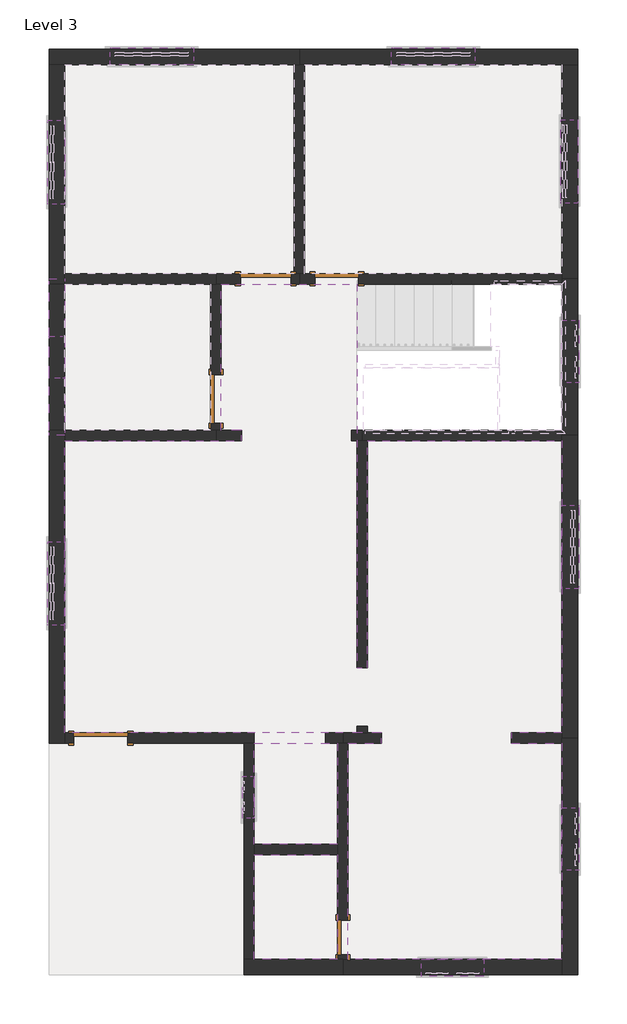
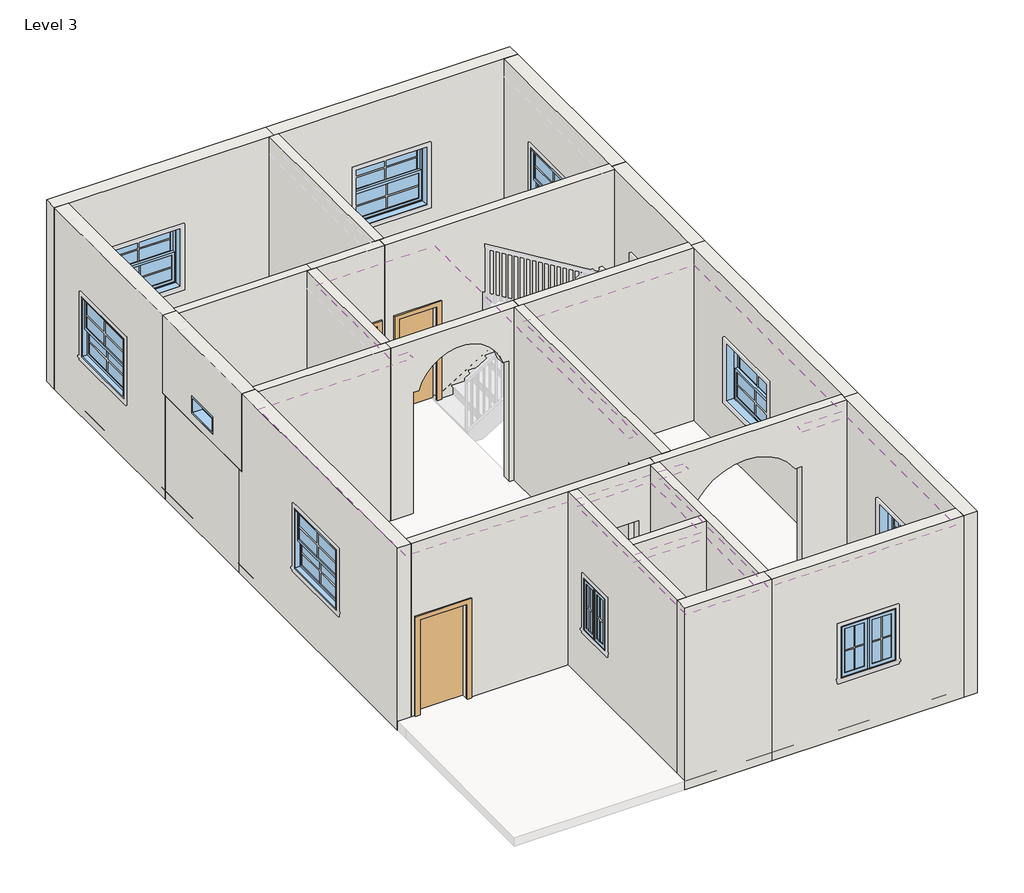
# One storey, part 1 of 2: 26 walls, 11 windows, 5 doors, 3 coverings.
# Revit data of these elements (continued)
# Element 15 (IfcWall, "Generic - 6\"")
#   built-in parameter 1001111 = 0' - 6"
#   Top Offset = 0' - 0"
#   Base Offset = 0' - 6"
#   Unconnected Height = 10' - 6"
#   wall height = 10' - 6"
#   Phase Created = New Construction
#   Base Constraint = Level 3
#   Materials on its faces: "Default Wall", "GOLD"
# Element 18 (IfcWall, "Generic - 6\"")
#   built-in parameter 1001111 = 0' - 6"
#   Top Offset = 0' - 0"
#   Base Offset = 0' - 6"
#   Unconnected Height = 10' - 6"
#   wall height = 10' - 6"
#   Phase Created = New Construction
#   Base Constraint = Level 3
#   Materials on its faces: "Default Wall", "DINING ROOM WALL", "LAVENDER WHITE"
# Elements 19, 21 (IfcWall, "Generic - 6\"")
#   built-in parameter 1001111 = 0' - 6"
#   Top Offset = 0' - 0"
#   Base Offset = 0' - 6"
#   Unconnected Height = 10' - 6"
#   wall height = 10' - 6"
#   Phase Created = New Construction
#   Base Constraint = Level 3
#   Materials on its faces: "Default Wall", "DINING ROOM WALL"
# Element 20 (IfcWall, "Generic - 6\"")
#   built-in parameter 1001111 = 0' - 6"
#   Top Offset = 0' - 0"
#   Base Offset = 0' - 6"
#   Unconnected Height = 10' - 6"
#   wall height = 10' - 6"
#   Phase Created = New Construction
#   Base Constraint = Level 3
#   Materials on its faces: "Default Wall", "LIVING ROOM WALL"
# Element 23 (IfcWall, "Generic - 9\"")
#   built-in parameter 1001111 = 0' - 6"
#   Top Offset = 0' - 0"
#   Base Offset = 0' - 6"
#   Unconnected Height = 10' - 6"
#   wall height = 10' - 6"
#   Phase Created = New Construction
#   Base Constraint = Level 3
#   Materials on its faces: "Default Wall", "BURGUNDY COLOUR"
# Elements 24, 26 (IfcWall, "Generic - 9\"")
#   built-in parameter 1001111 = 0' - 6"
#   Top Offset = 0' - 0"
#   Base Offset = 0' - 6"
#   Unconnected Height = 10' - 6"
#   wall height = 10' - 6"
#   Phase Created = New Construction
#   Base Constraint = Level 3
#   Materials on its faces: "Default Wall", "LAVENDER WHITE"
# Element 25 (IfcWall, "Generic - 9\"")
#   built-in parameter 1001111 = 0' - 6"
#   Top Offset = 0' - 0"
#   Base Offset = 0' - 6"
#   Unconnected Height = 10' - 6"
#   wall height = 10' - 6"
#   Phase Created = New Construction
#   Base Constraint = Level 3
#   Materials on its faces: "Default Wall", "GOLD"
# Elements 27, 28, 29, 31, 32 (IfcWall, "Generic - 9\"")
#   built-in parameter 1001111 = 0' - 6"
#   Top Offset = 0' - 0"
#   Base Offset = 0' - 6"
#   Unconnected Height = 10' - 6"
#   wall height = 10' - 6"
#   Phase Created = New Construction
#   Base Constraint = Level 3
#   Materials on its faces: "Default Wall"
# Element 30 (IfcWall, "Generic - 9\"")
#   built-in parameter 1001111 = 0' - 6"
#   Top Offset = 0' - 0"
#   Base Offset = 0' - 6"
#   Unconnected Height = 10' - 6"
#   wall height = 10' - 6"
#   Phase Created = New Construction
#   Base Constraint = Level 3
#   Materials on its faces: "Default Wall", "DINING ROOM WALL"
# Element 33 (IfcWall, "Generic - 9\"")
#   built-in parameter 1001111 = 6' - 6"
#   Top Offset = 0' - 0"
#   Base Offset = 6' - 6"
#   Unconnected Height = 4' - 6"
#   wall height = 4' - 6"
#   Phase Created = New Construction
#   Base Constraint = Level 3
#   Materials on its faces: "Default Wall", "BATHROOM TILES"
# Element 34 (IfcWall, "Generic - 9\"")
#   built-in parameter 1001111 = 0' - 6"
#   Top Offset = 0' - 0"
#   Base Offset = 0' - 6"
#   Unconnected Height = 6' - 0"
#   wall height = 6' - 0"
#   Phase Created = New Construction
#   Base Constraint = Level 3
#   Materials on its faces: "Default Wall", "BATHROOM TILES"
# Element 35 (IfcWindow, "Fixed : 2'")
#   Mark = "32"
#   Phase Created = New Construction
#   Materials on its faces: "Sash", "Glass"
# Element 36 (IfcWindow, "Window-Casement-Double : 2'")
#   Mark = "31"
#   Window Inset = 0' - 0"
#   Interior Wall Closure = 0' - 2 1/4"
#   Frame Extension = 0' - 0 1/4"
#   Exterior Wall Closure = 0' - 1 1/4"
#   Interior Trim Visibility = yes
#   Exterior Trim Visibility = yes
#   Phase Created = New Construction
#   Materials on its faces: "Wood - Stained", "Glass", "Clad - White"
# Element 37 (IfcWindow, "Window-Casement-Double : 3'")
#   Mark = "29"
#   Window Inset = 0' - 0"
#   Interior Wall Closure = 0' - 2 1/4"
#   Frame Extension = 0' - 0 1/4"
#   Exterior Wall Closure = 0' - 1 1/4"
#   Interior Trim Visibility = yes
#   Exterior Trim Visibility = yes
#   Phase Created = New Construction
#   Materials on its faces: "Wood - Stained", "Glass", "Clad - White"
# Element 38 (IfcWindow, "Window-Casement-Double : 3'")
#   Mark = "30"
#   Window Inset = 0' - 0"
#   Interior Wall Closure = 0' - 2 1/4"
#   Frame Extension = 0' - 0 1/4"
#   Exterior Wall Closure = 0' - 1 1/4"
#   Interior Trim Visibility = yes
#   Exterior Trim Visibility = yes
#   Phase Created = New Construction
#   Materials on its faces: "Wood - Stained", "Glass", "Clad - White"
# Element 39 (IfcWindow, "Window-Casement-Double : 3'")
#   Mark = "33"
#   Window Inset = 0' - 0"
#   Interior Wall Closure = 0' - 2 1/4"
#   Frame Extension = 0' - 0 1/4"
#   Exterior Wall Closure = 0' - 1 1/4"
#   Interior Trim Visibility = yes
#   Exterior Trim Visibility = yes
#   Phase Created = New Construction
#   Materials on its faces: "Wood - Stained", "Glass", "Clad - White"
# Element 40 (IfcWindow, "Window-Double-Hung : 4'")
#   Mark = "25"
#   Window Inset = 0' - 0"
#   Interior Wall Closure = 0' - 1 1/2"
#   Frame Extension = 0' - 1 1/4"
#   Exterior Wall Closure = 0' - 0 1/2"
#   Interior Trim Visibility = yes
#   Indicator Visibility = yes
#   Exterior Trim Visibility = yes
#   Phase Created = New Construction
#   Materials on its faces: "Wood - Stained", "Glass", "Clad - White"
# Element 41 (IfcWindow, "Window-Double-Hung : 4'")
#   Mark = "27"
#   Window Inset = 0' - 0"
#   Interior Wall Closure = 0' - 1 1/2"
#   Frame Extension = 0' - 1 1/4"
#   Exterior Wall Closure = 0' - 0 1/2"
#   Interior Trim Visibility = yes
#   Indicator Visibility = yes
#   Exterior Trim Visibility = yes
#   Phase Created = New Construction
#   Materials on its faces: "Wood - Stained", "Glass", "Clad - White"
# Element 42 (IfcWindow, "Window-Double-Hung : 4'")
#   Mark = "28"
#   Window Inset = 0' - 0"
#   Interior Wall Closure = 0' - 1 1/2"
#   Frame Extension = 0' - 1 1/4"
#   Exterior Wall Closure = 0' - 0 1/2"
#   Interior Trim Visibility = yes
#   Indicator Visibility = yes
#   Exterior Trim Visibility = yes
#   Phase Created = New Construction
#   Materials on its faces: "Wood - Stained", "Glass", "Clad - White"
# Element 43 (IfcWindow, "Window-Double-Hung : 4'")
#   Mark = "23"
#   Window Inset = 0' - 0"
#   Interior Wall Closure = 0' - 1 1/2"
#   Frame Extension = 0' - 1 1/4"
#   Exterior Wall Closure = 0' - 0 1/2"
#   Interior Trim Visibility = yes
#   Indicator Visibility = yes
#   Exterior Trim Visibility = yes
#   Phase Created = New Construction
#   Materials on its faces: "Wood - Stained", "Glass", "Clad - White"
# Element 44 (IfcWindow, "Window-Double-Hung : 4'")
#   Mark = "24"
#   Window Inset = 0' - 0"
#   Interior Wall Closure = 0' - 1 1/2"
#   Frame Extension = 0' - 1 1/4"
#   Exterior Wall Closure = 0' - 0 1/2"
#   Interior Trim Visibility = yes
#   Indicator Visibility = yes
#   Exterior Trim Visibility = yes
#   Phase Created = New Construction
#   Materials on its faces: "Wood - Stained", "Glass", "Clad - White"
# Element 45 (IfcWindow, "Window-Double-Hung : 4'")
#   Mark = "26"
#   Window Inset = 0' - 0"
#   Interior Wall Closure = 0' - 1 1/2"
#   Frame Extension = 0' - 1 1/4"
#   Exterior Wall Closure = 0' - 0 1/2"
#   Interior Trim Visibility = yes
#   Indicator Visibility = yes
#   Exterior Trim Visibility = yes
#   Phase Created = New Construction
#   Materials on its faces: "Wood - Stained", "Glass", "Clad - White"
# Materials
#   "Default": colour RGB 127 127 127, transparency 0, Cost = 0
#   "Acoustic Ceiling Tile 24 x 48": class "Generic", colour RGB 229 229 229, transparency 0, Description = "Acoustic Ceiling Tile 24 x 48", Cost = 0
#   "Door - Panel": class "Wood", colour RGB 210 159 95, transparency 0, Cost = 0
#   "Door - Frame": colour RGB 118 70 51, transparency 0, Cost = 0
#   "Glass": class "Glass", colour RGB 0 128 192, transparency 0.75, Description = "Soda Lime Glass", Cost = 0
#   "Sash": class "Wood", colour RGB 224 178 126, transparency 0, Cost = 0
#   "Wood - Stained": class "Wood", colour RGB 224 178 126, transparency 0, Cost = 0
#   "Clad - White": class "Wood", colour RGB 242 242 238, transparency 0, Cost = 0
#   "Default Wall": colour RGB 128 128 128, transparency 0, Cost = 0
#   "LAVENDER WHITE": class "Generic", colour RGB 120 120 120, transparency 0, Cost = 0
#   "LIVING ROOM WALL": class "Generic", colour RGB 120 120 120, transparency 0, Cost = 0
#   "BURGUNDY COLOUR": class "Generic", colour RGB 120 120 120, transparency 0, Cost = 0
#   "DINING ROOM WALL": class "Generic", colour RGB 120 120 120, transparency 0, Cost = 0
#   "GOLD": class "Generic", colour RGB 120 120 120, transparency 0, Cost = 0
#   "BATHROOM TILES": class "Generic", colour RGB 120 120 120, transparency 0, Cost = 0
